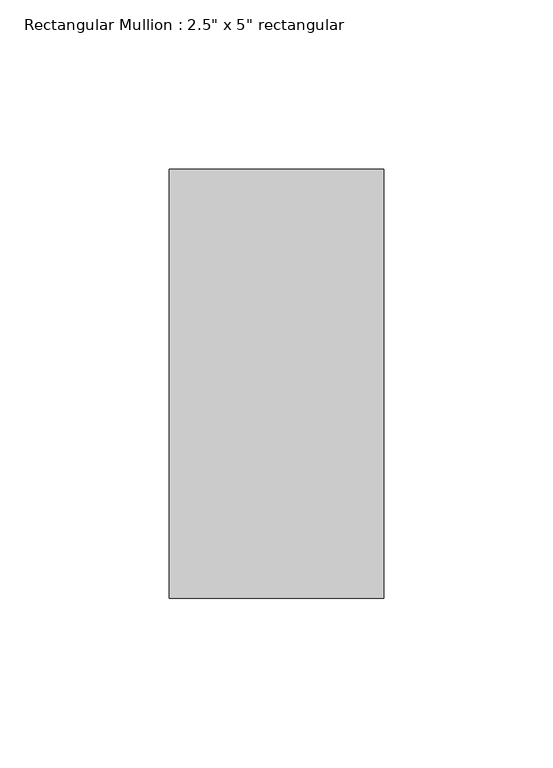
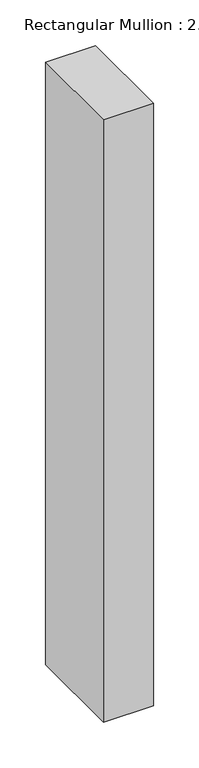
"""IFC4 building model written with IfcOpenShell, lengths in millimetres: member geometry."""

from ifc_helpers import new_model, si_unit, frame, origin, place, context, project, spatial, polyline, outline, extrude, source, transform, mapped, element, save


def member_70242a31(model_context):
    return source(origin(), model_context, "Body", "SweptSolid", [
        extrude(outline(polyline([(0.0, 63.5), (0.0, -63.5), (-63.5, -63.5), (-63.5, 63.5), (0.0, 63.5)])), frame((0.0, 0.0, -806.45), z_axis=(0.0, 0.0, 1.0), x_axis=(1.0, 0.0, 0.0)), (0.0, 0.0, 1.0), 806.45),
    ])


if __name__ == "__main__":
    model = new_model("IFC4")
    model_context = context("Model", 3, world=origin())
    ifc_project = project(units=[si_unit("LENGTHUNIT", "METRE", prefix="MILLI")], contexts=[model_context])
    site = spatial("IfcSite", under=ifc_project)
    building = spatial("IfcBuilding", under=site)
    placement = place(None, origin())
    member_shape = member_70242a31(model_context)
    element("IfcMember", 1, ObjectType="Rectangular Mullion : 2.5\" x 5\" rectangular", at=placement, inside=building, context=model_context, shape_type="MappedRepresentation", body=[
        mapped(member_shape, transform((0.0, 0.0, 0.0), x_axis=(1.0, 0.0, 0.0), y_axis=(0.0, 1.0, 0.0), z_axis=(0.0, 0.0, 1.0))),
    ])
    save(model, "model.ifc")

# Revit data of these elements
# Type "Rectangular Mullion : 2.5\" x 5\" rectangular"
#   built-in parameter 1007304 = 0.416667 (stored number, unit not read)
#   built-in parameter 1007301 = 0.104167 (stored number, unit not read)
#   built-in parameter 1007300 = 0.104167 (stored number, unit not read)
# Element 1 (IfcMember, "Rectangular Mullion : 2.5\" x 5\" rectangular")
#   Materials on its faces: "Aluminum"
# Materials
#   "Aluminum": class "Metal", colour RGB 247 247 247, transparency 0, Description = "Aluminum 6061", Cost = 0
